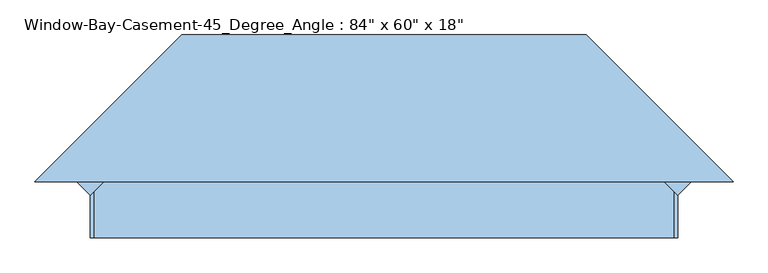
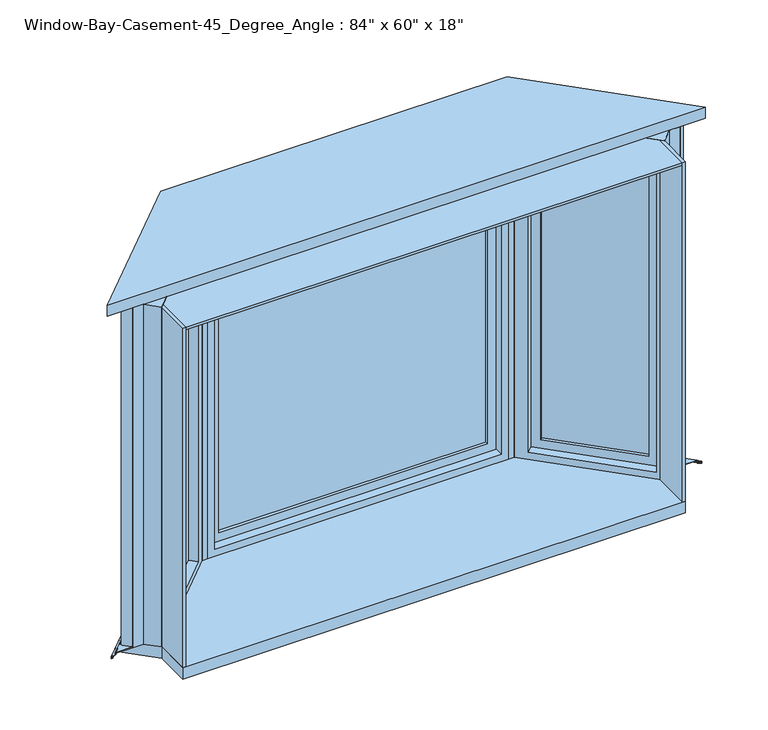
"""IFC4 building model written with IfcOpenShell, lengths in millimetres: window geometry."""

from ifc_helpers import new_model, si_unit, frame, origin, place, context, project, spatial, polyline, outline, extrude, faceted_brep, source, transform, mapped, element, save


def window_9f89e8e4(model_context):
    return source(origin(), model_context, "Body", "SolidModel", [
        extrude(outline(polyline([(1066.8, 150.9914087), (1062.3098719, 146.5012806), (771.5637138, 437.2474388), (776.0538418, 441.7375668), (1066.8, 150.9914087)])), frame((0.0, 0.0, 730.25), z_axis=(0.0, 0.0, 1.0), x_axis=(1.0, 0.0, 0.0)), (0.0, 0.0, 1.0), 1384.3),
        extrude(outline(polyline([(1057.8197439, 142.0111525), (1053.3296158, 137.5210245), (762.5834576, 428.2671827), (767.0735857, 432.7573107), (1057.8197439, 142.0111525)])), frame((0.0, 0.0, 730.25), z_axis=(0.0, 0.0, 1.0), x_axis=(1.0, 0.0, 0.0)), (0.0, 0.0, 1.0), 1384.3),
        extrude(outline(polyline([(1441.45, 57.15), (1441.45, -468.3271601), (-57.15, -468.3271601), (-57.15, 57.15), (1441.45, 57.15)]), holes=[polyline([(1384.3, -411.1771601), (1384.3, 0.0), (0.0, 0.0), (0.0, -411.1771601), (1384.3, -411.1771601)])]), frame((1044.3493597, 128.5407684, 730.25), z_axis=(0.7071067811865468, 0.7071067811865483, 0.0), x_axis=(0.0, 0.0, 1.0)), (0.0, 0.0, 1.0), 44.45),
        faceted_brep([(661.8085913, 457.2, 2184.4), (1066.8, 52.2085913, 2184.4), (1116.1914087, 101.6, 2184.4), (1161.0926893, 101.6, 2184.4), (703.8926893, 558.8, 2184.4), (1084.7605122, 88.1296158, 2171.7), (713.192049, 459.6980791, 2171.7), (758.0933296, 504.5993597, 2171.7), (1129.6617928, 133.0308964, 2171.7), (1044.3493597, 74.6592316, 2152.65), (699.7216648, 419.2869265, 2152.65), (726.6624332, 446.2276949, 2152.65), (1071.2901281, 101.6, 2152.65), (713.192049, 459.6980791, 673.1), (758.0933296, 504.5993597, 673.1), (699.7216648, 419.2869265, 692.15), (726.6624332, 446.2276949, 692.15), (703.8926893, 558.8, 660.4), (1161.0926893, 101.6, 660.4), (1116.1914087, 101.6, 660.4), (1066.8, 52.2085913, 660.4), (661.8085913, 457.2, 660.4), (1084.7605122, 88.1296158, 673.1), (1129.6617928, 133.0308964, 673.1), (1044.3493597, 74.6592316, 692.15), (1071.2901281, 101.6, 692.15)], [[[0, 1, 2, 3, 4]], [[5, 6, 7, 8]], [[9, 10, 11, 12]], [[6, 13, 14, 7]], [[10, 15, 16, 11]], [[17, 18, 19, 20, 21]], [[13, 22, 23, 14]], [[15, 24, 25, 16]], [[20, 19, 2, 1]], [[3, 18, 17, 4], [7, 14, 23, 8]], [[8, 23, 22, 5]], [[5, 22, 13, 6], [11, 16, 25, 12]], [[12, 25, 24, 9]], [[1, 0, 21, 20], [9, 24, 15, 10]], [[4, 17, 21, 0]], [[2, 19, 18, 3]]]),
        extrude(outline(polyline([(-1066.8, 150.9914087), (-776.0538418, 441.7375668), (-771.5637138, 437.2474388), (-1062.3098719, 146.5012806), (-1066.8, 150.9914087)])), frame((0.0, 0.0, 730.25), z_axis=(0.0, 0.0, 1.0), x_axis=(1.0, 0.0, 0.0)), (0.0, 0.0, 1.0), 1384.3),
        extrude(outline(polyline([(-1057.8197439, 142.0111525), (-767.0735857, 432.7573107), (-762.5834576, 428.2671827), (-1053.3296158, 137.5210245), (-1057.8197439, 142.0111525)])), frame((0.0, 0.0, 730.25), z_axis=(0.0, 0.0, 1.0), x_axis=(1.0, 0.0, 0.0)), (0.0, 0.0, 1.0), 1384.3),
        extrude(outline(polyline([(1441.45, -57.15), (-57.15, -57.15), (-57.15, 468.3271601), (1441.45, 468.3271601), (1441.45, -57.15)]), holes=[polyline([(1384.3, 411.1771601), (0.0, 411.1771601), (0.0, 0.0), (1384.3, 0.0), (1384.3, 411.1771601)])]), frame((-1044.3493597, 128.5407684, 730.25), z_axis=(-0.7071067811865468, 0.7071067811865483, 0.0), x_axis=(0.0, 0.0, 1.0)), (0.0, 0.0, 1.0), 44.45),
        faceted_brep([(-661.8085913, 457.2, 2184.4), (-703.8926893, 558.8, 2184.4), (-1161.0926893, 101.6, 2184.4), (-1116.1914087, 101.6, 2184.4), (-1066.8, 52.2085913, 2184.4), (-1084.7605122, 88.1296158, 2171.7), (-1129.6617928, 133.0308964, 2171.7), (-758.0933296, 504.5993597, 2171.7), (-713.192049, 459.6980791, 2171.7), (-1044.3493597, 74.6592316, 2152.65), (-1071.2901281, 101.6, 2152.65), (-726.6624332, 446.2276949, 2152.65), (-699.7216648, 419.2869265, 2152.65), (-758.0933296, 504.5993597, 673.1), (-713.192049, 459.6980791, 673.1), (-726.6624332, 446.2276949, 692.15), (-699.7216648, 419.2869265, 692.15), (-703.8926893, 558.8, 660.4), (-661.8085913, 457.2, 660.4), (-1066.8, 52.2085913, 660.4), (-1116.1914087, 101.6, 660.4), (-1161.0926893, 101.6, 660.4), (-1129.6617928, 133.0308964, 673.1), (-1084.7605122, 88.1296158, 673.1), (-1071.2901281, 101.6, 692.15), (-1044.3493597, 74.6592316, 692.15)], [[[0, 1, 2, 3, 4]], [[5, 6, 7, 8]], [[9, 10, 11, 12]], [[8, 7, 13, 14]], [[12, 11, 15, 16]], [[17, 18, 19, 20, 21]], [[14, 13, 22, 23]], [[16, 15, 24, 25]], [[19, 4, 3, 20]], [[2, 1, 17, 21], [7, 6, 22, 13]], [[6, 5, 23, 22]], [[5, 8, 14, 23], [11, 10, 24, 15]], [[10, 9, 25, 24]], [[4, 19, 18, 0], [9, 12, 16, 25]], [[1, 0, 18, 17]], [[3, 2, 21, 20]]]),
        faceted_brep([(-724.9347382, 609.6, 660.4), (-724.9347382, 609.6, 653.0697935), (724.9347382, 609.6, 653.0697935), (724.9347382, 609.6, 660.4), (-703.8926893, 558.8, 663.1486341), (-703.8926893, 558.8, 660.4), (703.8926893, 558.8, 660.4), (703.8926893, 558.8, 663.1486341), (-725.5133946, 610.997, 654.4483503), (-725.5133946, 610.997, 663.1486341), (725.5133946, 610.997, 663.1486341), (725.5133946, 610.997, 654.4483503), (730.7739068, 623.697, 652.2089977), (-730.7739068, 623.697, 652.2089977), (730.7739068, 623.697, 643.2668038), (-730.7739068, 623.697, 643.2668038), (-729.132627, 619.7346, 644.7270038), (-729.132627, 619.7346, 643.2668038), (729.132627, 619.7346, 643.2668038), (729.132627, 619.7346, 644.7270038), (-730.1110823, 622.0968, 650.8662705), (-730.1110823, 622.0968, 644.7270038), (730.1110823, 622.0968, 644.7270038), (730.1110823, 622.0968, 650.8662705), (-1232.9347382, 101.6, 660.4), (-1232.9347382, 101.6, 653.0697935), (1232.9347382, 101.6, 660.4), (1161.0926893, 101.6, 660.4), (-1161.0926893, 101.6, 660.4), (-1161.0926893, 101.6, 663.1486341), (1161.0926893, 101.6, 663.1486341), (1234.9103945, 101.6, 663.1486341), (-1234.9103945, 101.6, 663.1486341), (-1234.9103945, 101.6, 654.4483503), (-1252.8709068, 101.6, 652.2089977), (-1252.8709068, 101.6, 643.2668038), (1252.8709068, 101.6, 643.2668038), (1247.2672271, 101.6, 643.2668038), (-1247.2672271, 101.6, 643.2668038), (-1247.2672271, 101.6, 644.7270038), (1247.2672271, 101.6, 644.7270038), (1250.6078823, 101.6, 644.7270038), (-1250.6078823, 101.6, 644.7270038), (-1250.6078823, 101.6, 650.8662705), (1232.9347382, 101.6, 653.0697935), (1234.9103945, 101.6, 654.4483503), (1252.8709068, 101.6, 652.2089977), (1250.6078823, 101.6, 650.8662705)], [[[0, 1, 2, 3]], [[4, 5, 6, 7]], [[8, 9, 10, 11]], [[8, 11, 12, 13]], [[13, 12, 14, 15]], [[16, 17, 18, 19]], [[20, 21, 22, 23]], [[2, 1, 20, 23]], [[1, 0, 24, 25]], [[0, 3, 26, 27, 6, 5, 28, 24]], [[5, 4, 29, 28]], [[4, 7, 30, 31, 10, 9, 32, 29]], [[9, 8, 33, 32]], [[8, 13, 34, 33]], [[13, 15, 35, 34]], [[15, 14, 36, 37, 18, 17, 38, 35]], [[17, 16, 39, 38]], [[16, 19, 40, 41, 22, 21, 42, 39]], [[21, 20, 43, 42]], [[20, 1, 25, 43]], [[3, 2, 44, 26]], [[7, 6, 27, 30]], [[11, 10, 31, 45]], [[12, 11, 45, 46]], [[14, 12, 46, 36]], [[19, 18, 37, 40]], [[23, 22, 41, 47]], [[2, 23, 47, 44]], [[25, 24, 28, 29, 32, 33, 34, 35, 38, 39, 42, 43]], [[27, 26, 44, 47, 41, 40, 37, 36, 46, 45, 31, 30]]]),
        extrude(outline(polyline([(-1138.642049, 124.0506403), (-1161.0926893, 101.6), (-1192.5235857, 133.0308964), (-1170.0729454, 155.4815367), (-1138.642049, 124.0506403)])), frame((0.0, 0.0, 663.1486341), z_axis=(0.0, 0.0, 1.0), x_axis=(1.0, 0.0, 0.0)), (0.0, 0.0, 1.0), 1521.2513659),
        extrude(outline(polyline([(1138.642049, 124.0506403), (1170.0729454, 155.4815367), (1192.5235857, 133.0308964), (1161.0926893, 101.6), (1138.642049, 124.0506403)])), frame((0.0, 0.0, 663.1486341), z_axis=(0.0, 0.0, 1.0), x_axis=(1.0, 0.0, 0.0)), (0.0, 0.0, 1.0), 1521.2513659),
        extrude(outline(polyline([(735.4557627, 635.0), (1268.8557627, 101.6), (-1268.8557627, 101.6), (-735.4557627, 635.0), (735.4557627, 635.0)])), frame((0.0, 0.0, 2184.4), z_axis=(0.0, 0.0, 1.0), x_axis=(1.0, 0.0, 0.0)), (0.0, 0.0, 1.0), 50.8),
        extrude(outline(polyline([(-639.9414087, 558.8), (-639.9414087, 457.2), (-661.8085913, 457.2), (-703.8926893, 558.8), (-639.9414087, 558.8)])), frame((0.0, 0.0, 660.4), z_axis=(0.0, 0.0, 1.0), x_axis=(1.0, 0.0, 0.0)), (0.0, 0.0, 1.0), 1524.0),
        extrude(outline(polyline([(703.8926893, 558.8), (661.8085913, 457.2), (639.9414087, 457.2), (639.9414087, 558.8), (703.8926893, 558.8)])), frame((0.0, 0.0, 660.4), z_axis=(0.0, 0.0, 1.0), x_axis=(1.0, 0.0, 0.0)), (0.0, 0.0, 1.0), 1524.0),
        faceted_brep([(627.2414087, 495.3, 673.1), (627.2414087, 558.8, 673.1), (-627.2414087, 558.8, 673.1), (-627.2414087, 495.3, 673.1), (608.1914087, 457.2, 692.15), (608.1914087, 495.3, 692.15), (-608.1914087, 495.3, 692.15), (-608.1914087, 457.2, 692.15), (639.9414087, 558.8, 660.4), (639.9414087, 457.2, 660.4), (-639.9414087, 457.2, 660.4), (-639.9414087, 558.8, 660.4), (-627.2414087, 558.8, 2171.7), (-627.2414087, 495.3, 2171.7), (-608.1914087, 495.3, 2152.65), (-608.1914087, 457.2, 2152.65), (-639.9414087, 457.2, 2184.4), (-639.9414087, 558.8, 2184.4), (627.2414087, 558.8, 2171.7), (627.2414087, 495.3, 2171.7), (608.1914087, 495.3, 2152.65), (608.1914087, 457.2, 2152.65), (639.9414087, 457.2, 2184.4), (639.9414087, 558.8, 2184.4)], [[[0, 1, 2, 3]], [[4, 5, 6, 7]], [[8, 9, 10, 11]], [[3, 2, 12, 13]], [[7, 6, 14, 15]], [[11, 10, 16, 17]], [[13, 12, 18, 19]], [[15, 14, 20, 21]], [[17, 16, 22, 23]], [[11, 17, 23, 8], [1, 18, 12, 2]], [[19, 18, 1, 0]], [[3, 13, 19, 0], [5, 20, 14, 6]], [[21, 20, 5, 4]], [[9, 22, 16, 10], [7, 15, 21, 4]], [[23, 22, 9, 8]]]),
        extrude(outline(polyline([(570.0914087, 527.05), (570.0914087, 520.7), (-570.0914087, 520.7), (-570.0914087, 527.05), (570.0914087, 527.05)])), frame((0.0, 0.0, 730.25), z_axis=(0.0, 0.0, 1.0), x_axis=(1.0, 0.0, 0.0)), (0.0, 0.0, 1.0), 1384.3),
        extrude(outline(polyline([(570.0914087, 514.35), (570.0914087, 508.0), (-570.0914087, 508.0), (-570.0914087, 514.35), (570.0914087, 514.35)])), frame((0.0, 0.0, 730.25), z_axis=(0.0, 0.0, 1.0), x_axis=(1.0, 0.0, 0.0)), (0.0, 0.0, 1.0), 1384.3),
        extrude(outline(polyline([(1066.8, -101.6), (-1066.8, -101.6), (-1066.8, 52.2085913), (-1174.5630735, 159.9716648), (-724.9347382, 609.6), (724.9347382, 609.6), (1174.5630735, 159.9716648), (1066.8, 52.2085913), (1066.8, -101.6)])), frame((0.0, 0.0, 609.6), z_axis=(0.0, 0.0, 1.0), x_axis=(1.0, 0.0, 0.0)), (0.0, 0.0, 1.0), 50.8),
        extrude(outline(polyline([(2171.7, -627.2414087), (673.1, -627.2414087), (673.1, 627.2414087), (2171.7, 627.2414087), (2171.7, -627.2414087)]), holes=[polyline([(2114.55, 570.0914087), (730.25, 570.0914087), (730.25, -570.0914087), (2114.55, -570.0914087), (2114.55, 570.0914087)])]), frame((0.0, 495.3, 0.0), z_axis=(0.0, 1.0, 0.0), x_axis=(0.0, 0.0, 1.0)), (0.0, 0.0, 1.0), 44.45),
        extrude(outline(polyline([(-1066.8, -101.6), (-1066.8, 52.2085913), (-1054.1, 64.9085913), (-1054.1, -101.6), (-1066.8, -101.6)])), frame((0.0, 0.0, 660.4), z_axis=(0.0, 0.0, 1.0), x_axis=(1.0, 0.0, 0.0)), (0.0, 0.0, 1.0), 1524.0),
        extrude(outline(polyline([(1066.8, -101.6), (1054.1, -101.6), (1054.1, 64.9085913), (1066.8, 52.2085913), (1066.8, -101.6)])), frame((0.0, 0.0, 660.4), z_axis=(0.0, 0.0, 1.0), x_axis=(1.0, 0.0, 0.0)), (0.0, 0.0, 1.0), 1524.0),
        extrude(outline(polyline([(-661.8085913, 457.2), (661.8085913, 457.2), (1054.1, 64.9085913), (1054.1, -101.6), (-1054.1, -101.6), (-1054.1, 64.9085913), (-661.8085913, 457.2)])), frame((0.0, 0.0, 2171.7), z_axis=(0.0, 0.0, 1.0), x_axis=(1.0, 0.0, 0.0)), (0.0, 0.0, 1.0), 12.7),
    ])


if __name__ == "__main__":
    model = new_model("IFC4")
    model_context = context("Model", 3, world=origin())
    ifc_project = project(units=[si_unit("LENGTHUNIT", "METRE", prefix="MILLI")], contexts=[model_context])
    site = spatial("IfcSite", under=ifc_project)
    building = spatial("IfcBuilding", under=site)
    placement = place(None, origin())
    window_shape = window_9f89e8e4(model_context)
    element("IfcWindow", 1, ObjectType="Window-Bay-Casement-45_Degree_Angle : 84\" x 60\" x 18\"", at=placement, inside=building, context=model_context, shape_type="MappedRepresentation", body=[
        mapped(window_shape, transform((0.0, 0.0, 0.0), x_axis=(1.0, 0.0, 0.0), y_axis=(0.0, 1.0, 0.0), z_axis=(0.0, 0.0, 1.0))),
    ])
    save(model, "model.ifc")

# Revit data of these elements
# Type "Window-Bay-Casement-45_Degree_Angle : 84\" x 60\" x 18\""
#   Type Mark = "18"
#   Fire Rating = "0.5h"
#   Assembly Code = "B2020100"
#   Analytic Construction = "Double glazing - domestic"
#   Width of Middle Sash = 4' - 2.38909"
#   Width = 7' - 0"
#   Visual Light Transmittance = 0.81
#   Thermal Resistance (R) = 1.8146 (h·ft²·°F)/BTU
#   Solar Heat Gain Coefficient = 0.76
#   Rough Width = 7' - 0 1/2"
#   Rough Height = 5' - 0 1/2"
#   Length 4 = 0' - 1.13909"
#   Length 3 = 0' - 0.51777"
#   Length 2 = 4' - 7.42462"
#   Length 1 = 1' - 2.80546"
#   Wall Thickness [instance default] = 0' - 6"
#   Trim Width = 7' - 5.03553"
#   Trim Height = 5' - 0"
#   Height 1 = 5' - 2"
#   Height = 5' - 0"
#   Heat Transfer Coefficient (U) = 0.5511 BTU/(h·ft²·°F)
#   Depth = 1' - 6"
#   Default Sill Height = 2' - 0"
#   Angle 1 = 22.50°
#   Angle = 45.00°
#   Center Muntin Visibility = yes
#   Side Muntin Visibility = yes
#   Interior Trim Visibility [instance default] = yes
#   Exterior Trim Visibility [instance default] = yes
#   Center Muntin Pattern = Muntin Pattern_2x2 : Muntin Pattern_2x2
#   Side Muntin Pattern = Muntin Pattern_2x2 : Muntin Pattern_2x2
#   Interior Trim Material = Wood - Stained
#   Exterior Trim Material = Clad - White
#   Exterior Trim = element 406231
#   Interior Trim = Trim-Window-Interior-Flat : Picture Frame
#   Interior Frame Material = Wood - Stained
#   Glass Panel Material = Glass
#   Exterior Frame Material = Clad - White
#   Wall Closure = (empty or 0)
# Element 1 (IfcWindow, "Window-Bay-Casement-45_Degree_Angle : 84\" x 60\" x 18\"")
#   Wall Thickness = 0' - 8"
#   Materials on its faces: "Wood - Stained", "Clad - White", "Glass"
# Materials
#   "Wood - Stained": class "Wood", colour RGB 224 178 126, transparency 0, Cost = 0
#   "Clad - White": class "Wood", colour RGB 242 242 238, transparency 0, Cost = 0
#   "Glass": class "Glass", colour RGB 0 128 192, transparency 0.75, Description = "Soda Lime Glass", Cost = 0
